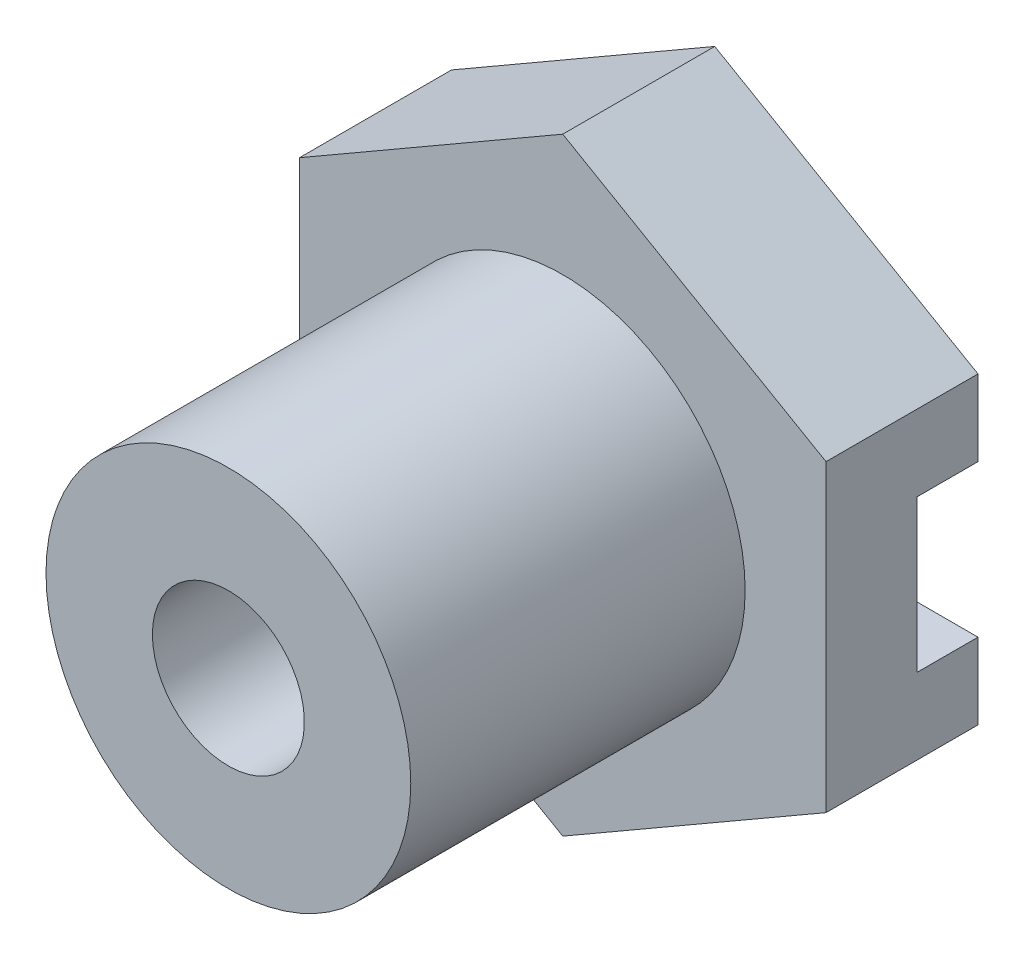
SolidWorks part; units mm, degrees
material "Plain Carbon Steel"
ref_plane "Front Plane" through (0, 0, 0) normal (0, 0, 1) x (1, 0, 0)
ref_plane "Top Plane" through (0, 0, 0) normal (0, 1, 0) x (1, 0, 0)
ref_plane "Right Plane" through (0, 0, 0) normal (1, 0, 0) x (0, 0, -1)
sketch "Hex Flange Sketch" plane through (0, 0, 0) normal (0, 0, 1) x (1, 0, 0)
  line L1 (0, 10) -> (-8.6603, 5)
  line L2 (-8.6603, 5) -> (-8.6603, -5)
  line L3 (-8.6603, -5) -> (0, -10)
  line L4 (0, -10) -> (8.6603, -5)
  line L5 (8.6603, -5) -> (8.6603, 5)
  line L6 (8.6603, 5) -> (0, 10)
  circle A0 centre (0, 0) radius 10 construction
  dimension "D1" = 20
extrude "Hex Flange" add sketch "Hex Flange Sketch" along normal blind 5
sketch "Boss Sketch Ø12" plane through (0, 0, 5) normal (0, 0, 1) x (1, 0, 0)
  circle A0 centre (0, 0) radius 6
  dimension "D1" = 12
extrude "Cylindrical Boss Ø12" add sketch "Boss Sketch Ø12" along normal blind 11
sketch "Flange Slot Sketch" plane through (0, 0, 0) normal (0, 0, -1) x (-1, 0, 0)
  line L0 (8.6603, 5) -> (8.6603, -5) construction
  line L1 (-8.6603, 2.5) -> (8.6603, 2.5)
  line L2 (-8.6603, 2.5) -> (-8.6603, -2.5)
  line L3 (-8.6603, -2.5) -> (8.6603, -2.5)
  line L4 (8.6603, 2.5) -> (8.6603, -2.5)
  line L5 (-8.6603, 2.5) -> (8.6603, -2.5) construction
  line L6 (-8.6603, -2.5) -> (8.6603, 2.5) construction
  point P0 (0, 0)
  dimension "D1" = 5
extrude "Flange Slot Cut" cut sketch "Flange Slot Sketch" against normal blind 2
sketch "Bore Sketch Ø5" plane through (0, 0, 2) normal (0, 0, -1) x (-1, 0, 0)
  circle A0 centre (0, 0) radius 2.5
  dimension "D1" = 5
extrude "Bore Ø5" cut sketch "Bore Sketch Ø5" against normal through all
